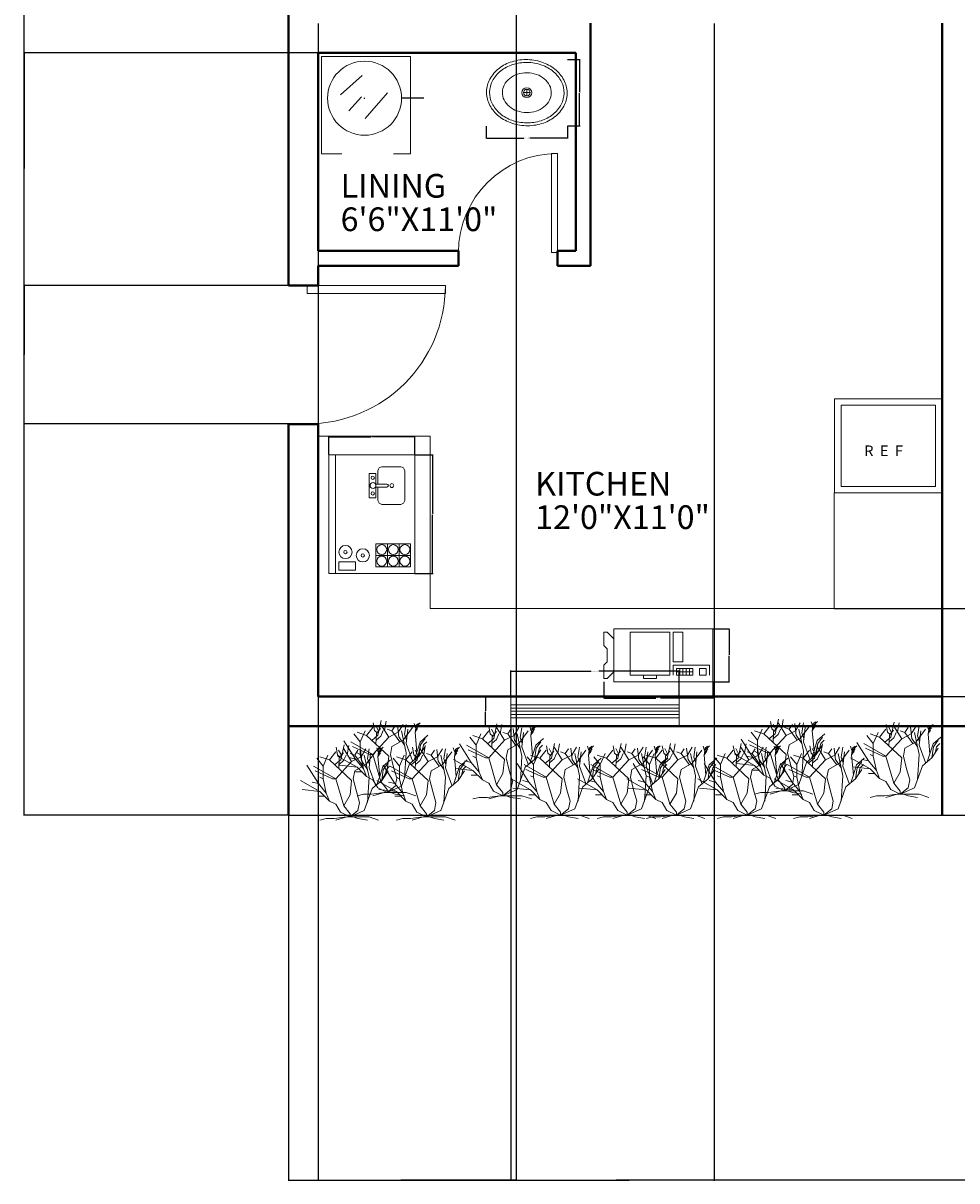
# Model space of a CAD drawing. Units: inches. Extents: x 12978 to 13669, y 46550 to 47327.
# Tile 1 of 5: x 12979 to 13262, y 46550 to 46901. Entities that reach past the tile are written whole.
import ezdxf

# ---------------------------------------------------------------- set-up
doc = ezdxf.new("R2010")
doc.units = ezdxf.units.IN
for name, color, linetype, lineweight in [('A-ANNO-DIMS', 2, 'Continuous', 18), ('A-AREA-IDEN', 1, 'Continuous', 18), ('A-EQPM', 8, 'Continuous', 18), ('A-FLOR-CASE', 8, 'Continuous', 20), ('A-FLOR-FIXT', 9, 'Continuous', 18), ('A-FLOR-OTLN', 7, 'Continuous', 25), ('door', 4, 'Continuous', 20), ('L-PLNT-TREE', 94, 'Continuous', 13), ('text', 1, 'Continuous', 18), ('wall', 7, 'Continuous', 40), ('window', 1, 'Continuous', 18)]:
    doc.layers.add(name, color=color, linetype=linetype, lineweight=lineweight)
doc.styles.get("Standard").update_dxf_attribs({"font": 'arial.ttf'})
doc.dimstyles.get("Standard").update_dxf_attribs({"dimtxt": 0.18, "dimasz": 0.18, "dimexe": 0.18, "dimexo": 0.0625, "dimgap": 0.09, "dimtad": 0, "dimtih": 1, "dimtoh": 1, "dimdec": 4, "dimzin": 0, "dimdsep": 46, "dimtxsty": 'Standard', "dimcen": 0.09, "dimadec": 0, "dimazin": 0, "dimtfac": 1, "dimtdec": 4, "dimtofl": 0, "dimtmove": 0, "dimatfit": 3, "dimfxl": 1, "dimtolj": 1, "dimtzin": 0, "dimarcsym": 0})

# ---------------------------------------------------------------- blocks, each defined once
blk = doc.blocks.new('*U2')
for p, q in [((0, 0), (0, -100)), ((750, 0), (750, -100))]:
    blk.add_line(p, q)
blk.add_lwpolyline([(0, 0), (0, 750), (43.75, 750), (43.75, 0)], close=True)
blk.add_arc((0, 0), 750, 0, 90)
blk = doc.blocks.new('Sink - Oval top')
for p, q in [((-1, 0), (1, 0)), ((0, 1), (0, -1))]:
    blk.add_line(p, q)
for points in [[(-12.23, 0.39, 0.117634), (-11.46, -3.36, 0.104469), (-8.88, -6.8, 0.090016), (-5.08, -9.07, 0.08192), (-0.32, -10.02, 0.08192), (4.49, -9.38, 0.090016), (8.42, -7.36, 0.104469), (11.22, -4.09, 0.117634), (12.23, -0.39, 0.117634), (11.46, 3.36, 0.104469), (8.88, 6.8, 0.090016), (5.08, 9.07, 0.08192), (0.32, 10.02, 0.08192), (-4.49, 9.38, 0.090016), (-8.42, 7.36, 0.104469), (-11.22, 4.09, 0.117634)], [(-11.29, 0.16, 0.118622), (-10.52, -3.25, 0.104678), (-8.07, -6.36, 0.089562), (-4.54, -8.37, 0.081185), (-0.13, -9.15, 0.081185), (4.3, -8.49, 0.089562), (7.89, -6.58, 0.104678), (10.42, -3.55, 0.118622), (11.29, -0.16, 0.118622), (10.52, 3.25, 0.104678), (8.07, 6.36, 0.089562), (4.54, 8.37, 0.081185), (0.13, 9.15, 0.081185), (-4.3, 8.49, 0.089562), (-7.89, 6.58, 0.104678), (-10.42, 3.55, 0.118622)], [(-7.42, 0.08, 0.118283), (-6.91, -2.17, 0.104607), (-5.29, -4.21, 0.089718), (-2.97, -5.53, 0.081436), (-0.07, -6.04, 0.081436), (2.84, -5.59, 0.089718), (5.2, -4.33, 0.104607), (6.86, -2.32, 0.118283), (7.42, -0.08, 0.118283), (6.91, 2.17, 0.104607), (5.29, 4.21, 0.089718), (2.97, 5.53, 0.081436), (0.07, 6.04, 0.081436), (-2.84, 5.59, 0.089718), (-5.2, 4.33, 0.104607), (-6.86, 2.32, 0.118283)]]:
    blk.add_lwpolyline(points, format="xyb", close=True)
for radius in [1.5, 1]:
    blk.add_circle((0, 0), radius)
blk = doc.blocks.new('Wet Bar')
for p, q in [((0, 0), (36, 0)), ((0, -26), (0, 0)), ((36, 0), (36, -26)), ((0, -2), (36, -2)), ((3.5, -3), (1, -3)), ((1, -3), (1, -8)), ((3.5, -8), (3.5, -3)), ((1, -8), (3.5, -8)), ((2, -14.25), (9, -14.25)), ((2, -24.75), (2, -14.25)), ((5.5, -14.25), (5.5, -24.75)), ((9, -14.25), (9, -24.75)), ((26.2, -17.55), (26.2, -14.1284)), ((27.1001, -17.55), (27.1001, -14.1284)), ((2, -17.75), (9, -17.75)), ((9, -21.25), (2, -21.25)), ((36, -26), (0, -26)), ((9, -24.75), (2, -24.75))]:
    blk.add_line(p, q)
for points in [[(26.2, -14.25), (22.95, -14.25), (22.95, -12.2), (26.75, -12.2)], [(26.7487, -12.2), (30.3501, -12.2), (30.3501, -14.25), (27.1001, -14.25)], [(20.95, -21.75), (20.95, -16.05)], [(22.15, -14.85), (26.2, -14.85)], [(27.1001, -14.85), (31.15, -14.85)], [(32.3501, -16.05), (32.3501, -21.75)], [(31.15, -22.95), (22.15, -22.95)]]:
    blk.add_lwpolyline(points)
for centre, radius in [((6.5, -5), 2), ((6.5, -5), 0.5), ((5.5, -10.25), 2), ((5.5, -10.25), 0.5), ((24.25, -13.25), 0.5), ((26.65, -13.35), 0.9), ((29, -13.25), 0.5), ((3.75, -16), 1.5), ((7.25, -16), 1.5), ((3.75, -19.5), 1.5), ((7.25, -19.5), 1.5), ((26.65, -19.05), 0.6), ((3.75, -23), 1.5), ((7.25, -23), 1.5)]:
    blk.add_circle(centre, radius)
for centre, radius, start, end in [((22.2251, -16.125), 1.2772, 93.36646, 176.6335), ((31.075, -16.125), 1.2772, 3.366461, 86.63354), ((26.65, -17.55), 0.45, 180, 0), ((22.2251, -21.675), 1.2772, 183.3665, 266.6335), ((31.075, -21.675), 1.2772, 273.3665, 356.6335)]:
    blk.add_arc(centre, radius, start, end)
blk = doc.blocks.new('Copy Machine')
for p, q in [((0, 0), (0, -16)), ((30, 0), (0, 0)), ((30, -16), (30, 0)), ((-3, -1), (-3, -5)), ((-2, -1), (-3, -1)), ((0, -3), (-2, -1)), ((5, -1), (5, -14)), ((17, -1), (5, -1)), ((17, -14), (17, -1)), ((18, -1), (18, -10)), ((21, -1), (18, -1)), ((21, -10), (21, -1)), ((-3, -5), (-2, -6)), ((-2, -10), (-2, -6)), ((-3, -11), (-2, -10)), ((18, -10), (21, -10)), ((-3, -15), (-3, -11)), ((0, -13), (-2, -15)), ((5, -14), (17, -14)), ((9, -14), (9, -15)), ((13, -15), (13, -14)), ((18, -14), (18, -11)), ((18, -11), (29, -11)), ((24, -12), (19, -12)), ((19, -12), (19, -14)), ((24, -13), (19, -13)), ((19, -14), (24, -14)), ((20, -12), (20, -14)), ((21, -14), (21, -12)), ((22, -12), (22, -14)), ((23, -14), (23, -12)), ((24, -14), (24, -12)), ((28, -12), (26, -12)), ((26, -12), (26, -14)), ((26, -14), (28, -14)), ((28, -14), (28, -12)), ((29, -11), (29, -14)), ((-2, -15), (-3, -15)), ((0, -16), (30, -16)), ((9, -15), (13, -15))]:
    blk.add_line(p, q)
blk = doc.blocks.new('*U13')
for p, q in [((-12.471, 19.775), (-12.898, 22.044)), ((-11.28, 19.619), (-12.104, 21.184)), ((-11.433, 18.289), (-10.457, 22.749)), ((-8.16, 17.76), (-10.56, 21.6)), ((-9.48, 19.775), (-8.992, 22.592)), ((-7.2, 19.68), (-6.24, 21.12)), ((-5.086, 17.741), (-5.513, 21.34)), ((-5.28, 19.2), (-3.84, 21.6)), ((-3.377, 18.602), (-2.888, 21.575)), ((-0.508, 21.888), (-0.081, 20.558)), ((-0.203, 19.149), (0.102, 21.34)), ((-0.02, 20.01), (0.896, 21.105)), ((0.041, 20.714), (1.384, 22.044)), ((0.102, 21.34), (0.835, 21.888)), ((-16.8, 16.32), (-18.72, 18.72)), ((-14.88, 18.24), (-17.76, 19.2)), ((-16.8, 16.32), (-15.36, 19.68)), ((-14.88, 18.24), (-12.96, 20.64)), ((-8.16, 12), (-14.88, 18.24)), ((-13.325, 16.724), (-11.433, 18.289)), ((-12.96, 12.48), (-8.16, 17.76)), ((-11.677, 19.071), (-12.471, 19.775)), ((-12.043, 15.628), (-11.921, 18.836)), ((-11.982, 16.802), (-10.579, 18.054)), ((-11.921, 18.836), (-10.64, 20.401)), ((-10.579, 18.054), (-9.846, 19.697)), ((-7.2, 19.68), (-8.64, 20.16)), ((-8.16, 17.76), (-5.28, 19.2)), ((-4.8, 16.32), (-7.2, 19.68)), ((-3.377, 15.315), (-5.086, 17.819)), ((-2.88, 12.96), (-4.32, 19.68)), ((-3.84, 16.8), (-0.96, 20.64)), ((-2.766, 16.802), (-3.377, 18.602)), ((-2.88, 15.84), (-2.4, 20.16)), ((0.346, 13.203), (-0.203, 19.149)), ((-0.142, 19.384), (0.59, 20.401)), ((1.323, 16.254), (3.642, 18.289)), ((-18.24, 11.04), (-21.755, 16.655)), ((-12.96, 12.48), (-19.68, 16.32)), ((-13.92, 12.48), (-19.2, 14.88)), ((-16.8, 12.48), (-16.8, 16.32)), ((-7.68, 12.48), (-7.2, 14.88)), ((-7.2, 14.88), (-3.84, 16.8)), ((-0.96, 10.56), (-2.88, 15.84)), ((0.346, 13.203), (1.323, 16.254)), ((0.96, 12), (1.44, 15.36)), ((0.96, 12), (2.88, 14.88)), ((1.44, 15.36), (2.88, 17.28)), ((1.92, 13.44), (2.4, 15.36)), ((2.4, 15.36), (3.36, 16.32)), ((-17.76, 8.64), (-23.663, 11.961)), ((-18.24, 11.04), (-20.16, 11.52)), ((-15.84, 8.16), (-18.24, 11.04)), ((-16.8, 12.48), (-17.76, 12.96)), ((-15.84, 8.16), (-16.8, 12.48)), ((-12.96, 12.48), (-13.92, 12.48)), ((-10.56, 4.32), (-12.96, 12.48)), ((-8.64, 7.68), (-8.16, 12)), ((-6.72, 8.64), (-7.68, 12.48)), ((-3.36, 5.28), (-2.88, 12.96)), ((-1.92, 9.6), (0.96, 12)), ((-0.48, 10.8), (0.346, 13.203)), ((-17.76, 8.64), (-23.128, 9.222)), ((-16.32, 7.2), (-18.24, 7.2)), ((-14.88, 5.76), (-17.76, 8.64)), ((-14.88, 5.76), (-15.84, 8.16)), ((-10.56, 4.32), (-8.64, 7.68)), ((-5.76, 5.28), (-6.72, 8.64)), ((-4.32, 2.88), (-1.92, 9.6)), ((-12.96, 4.8), (-14.88, 5.76)), ((-11.52, 2.4), (-12.96, 4.8)), ((-8.64, 1.92), (-10.56, 4.32)), ((-6.24, 2.88), (-5.76, 5.28)), ((-15.84, 0.48), (-17.76, 0)), ((-13.44, 0.48), (-15.84, 0.48)), ((-9.6, 0.96), (-13.44, 0.48)), ((-9.6, 0.96), (-12.96, 0)), ((-8.64, 0.96), (-11.52, 2.4)), ((-9.6, 0.96), (-7.68, 0.96)), ((-8.64, 0.96), (-4.32, 2.88)), ((-8.64, 0.96), (-6.24, 2.88)), ((-8.64, 0.96), (-8.64, 1.92)), ((-8.64, 0.96), (-2.88, 0.96)), ((-7.68, 0.96), (-6.24, 0.48)), ((-6.24, 0.48), (-3.36, 0)), ((-2.88, 0.96), (0, 0))]:
    blk.add_line(p, q)
blk = doc.blocks.new('WINDOW-51')
for p, q in [((0, 0), (0, 9)), ((51.08, 0), (51.08, 9)), ((0, 6.5), (51.08, 6.5)), ((0, 5.5), (51.08, 5.5)), ((0, 4.5), (51.08, 4.5)), ((0, 3.5), (51.08, 3.5)), ((0, 2.5), (51.08, 2.5))]:
    blk.add_line(p, q)
blk = doc.blocks.new('*D43')
at = {"layer": 'A-ANNO-DIMS', "color": 0, "lineweight": -2, "transparency": 16777216}
for p, q in [((13097.3, 46769.89), (13102.82, 46769.89)), ((13102.64, 46769.71), (13102.64, 46752.07)), ((13102.64, 46734.07), (13102.64, 46751.7)), ((13097.3, 46733.89), (13102.82, 46733.89))]:
    blk.add_line(p, q, dxfattribs=at)
at = {"layer": 'A-ANNO-DIMS', "color": 0, "transparency": 16777216}
for points in [[(13102.61, 46769.71), (13102.67, 46769.71), (13102.64, 46769.89)], [(13102.61, 46734.07), (13102.67, 46734.07), (13102.64, 46733.89)]]:
    blk.add_solid(points, dxfattribs=at)
at = {"layer": 'Defpoints', "color": 0, "transparency": 16777216}
for p in [(13097.24, 46769.89), (13102.64, 46769.89), (13097.24, 46733.89)]:
    blk.add_point(p, dxfattribs=at)
at = {"layer": 'A-ANNO-DIMS', "color": 0, "transparency": 16777216, "insert": (13102.64, 46751.89), "char_height": 0.18, "attachment_point": 5}
blk.add_mtext('\\A1;BAR 36', dxfattribs=at)
blk = doc.blocks.new('*D44')
at = {"layer": 'A-ANNO-DIMS', "color": 0, "lineweight": -2, "transparency": 16777216}
for p, q in [((13071.24, 46769.95), (13071.24, 46775.47)), ((13071.42, 46775.29), (13084.01, 46775.29)), ((13097.06, 46775.29), (13084.46, 46775.29)), ((13097.24, 46769.95), (13097.24, 46775.47))]:
    blk.add_line(p, q, dxfattribs=at)
at = {"layer": 'A-ANNO-DIMS', "color": 0, "transparency": 16777216}
for points in [[(13071.42, 46775.32), (13071.42, 46775.26), (13071.24, 46775.29)], [(13097.06, 46775.32), (13097.06, 46775.26), (13097.24, 46775.29)]]:
    blk.add_solid(points, dxfattribs=at)
at = {"layer": 'Defpoints', "color": 0, "transparency": 16777216}
for p in [(13071.24, 46775.29), (13071.24, 46769.89), (13097.24, 46769.89)]:
    blk.add_point(p, dxfattribs=at)
at = {"layer": 'A-ANNO-DIMS', "color": 0, "transparency": 16777216, "insert": (13084.24, 46775.29), "char_height": 0.18, "attachment_point": 5}
blk.add_mtext('\\A1;26', dxfattribs=at)
blk = doc.blocks.new('*D45')
at = {"layer": 'A-ANNO-DIMS', "color": 0, "lineweight": -2, "transparency": 16777216}
for p, q in [((13154.51, 46701.03), (13154.51, 46695.97)), ((13187.51, 46701.03), (13187.51, 46695.97)), ((13154.69, 46696.15), (13170.28, 46696.15)), ((13187.33, 46696.15), (13171.75, 46696.15))]:
    blk.add_line(p, q, dxfattribs=at)
at = {"layer": 'A-ANNO-DIMS', "color": 0, "transparency": 16777216}
for points in [[(13154.69, 46696.18), (13154.69, 46696.12), (13154.51, 46696.15)], [(13187.33, 46696.18), (13187.33, 46696.12), (13187.51, 46696.15)]]:
    blk.add_solid(points, dxfattribs=at)
at = {"layer": 'Defpoints', "color": 0, "transparency": 16777216}
for p in [(13154.51, 46701.1), (13187.51, 46701.1), (13187.51, 46696.15)]:
    blk.add_point(p, dxfattribs=at)
at = {"layer": 'A-ANNO-DIMS', "color": 0, "transparency": 16777216, "insert": (13171.01, 46696.15), "char_height": 0.18, "attachment_point": 5}
blk.add_mtext('\\A1;COPIER 33', dxfattribs=at)
blk = doc.blocks.new('*D46')
at = {"layer": 'A-ANNO-DIMS', "color": 0, "lineweight": -2, "transparency": 16777216}
for p, q in [((13187.57, 46717.1), (13192.64, 46717.1)), ((13192.46, 46716.92), (13192.46, 46709.28)), ((13192.46, 46701.28), (13192.46, 46708.91)), ((13187.57, 46701.1), (13192.64, 46701.1))]:
    blk.add_line(p, q, dxfattribs=at)
at = {"layer": 'A-ANNO-DIMS', "color": 0, "transparency": 16777216}
for points in [[(13192.43, 46716.92), (13192.49, 46716.92), (13192.46, 46717.1)], [(13192.43, 46701.28), (13192.49, 46701.28), (13192.46, 46701.1)]]:
    blk.add_solid(points, dxfattribs=at)
at = {"layer": 'Defpoints', "color": 0, "transparency": 16777216}
for p in [(13187.51, 46717.1), (13192.46, 46717.1), (13187.51, 46701.1)]:
    blk.add_point(p, dxfattribs=at)
at = {"layer": 'A-ANNO-DIMS', "color": 0, "transparency": 16777216, "insert": (13192.46, 46709.1), "char_height": 0.18, "attachment_point": 5}
blk.add_mtext('\\A1;16', dxfattribs=at)
blk = doc.blocks.new('*D47')
at = {"layer": 'A-ANNO-DIMS', "color": 0, "lineweight": -2, "transparency": 16777216}
for p, q in [((13118.92, 46869.44), (13118.92, 46865.64)), ((13143.47, 46869.44), (13143.47, 46865.64)), ((13119.1, 46865.82), (13130.26, 46865.82)), ((13143.29, 46865.82), (13132.13, 46865.82))]:
    blk.add_line(p, q, dxfattribs=at)
at = {"layer": 'A-ANNO-DIMS', "color": 0, "transparency": 16777216}
for points in [[(13119.1, 46865.85), (13119.1, 46865.79), (13118.92, 46865.82)], [(13143.29, 46865.85), (13143.29, 46865.79), (13143.47, 46865.82)]]:
    blk.add_solid(points, dxfattribs=at)
at = {"layer": 'Defpoints', "color": 0, "transparency": 16777216}
for p in [(13118.92, 46869.51), (13143.47, 46869.51), (13143.47, 46865.82)]:
    blk.add_point(p, dxfattribs=at)
at = {"layer": 'A-ANNO-DIMS', "color": 0, "transparency": 16777216, "insert": (13131.19, 46865.82), "char_height": 0.18, "attachment_point": 5}
blk.add_mtext('\\A1;BASIN 25 TYP.', dxfattribs=at)
blk = doc.blocks.new('*D48')
at = {"layer": 'A-ANNO-DIMS', "color": 0, "lineweight": -2, "transparency": 16777216}
for p, q in [((13143.53, 46889.64), (13147.33, 46889.64)), ((13147.15, 46889.46), (13147.15, 46879.76)), ((13147.15, 46869.69), (13147.15, 46879.39)), ((13143.53, 46869.51), (13147.33, 46869.51))]:
    blk.add_line(p, q, dxfattribs=at)
at = {"layer": 'A-ANNO-DIMS', "color": 0, "transparency": 16777216}
for points in [[(13147.12, 46889.46), (13147.18, 46889.46), (13147.15, 46889.64)], [(13147.12, 46869.69), (13147.18, 46869.69), (13147.15, 46869.51)]]:
    blk.add_solid(points, dxfattribs=at)
at = {"layer": 'Defpoints', "color": 0, "transparency": 16777216}
for p in [(13143.47, 46889.64), (13147.15, 46889.64), (13143.47, 46869.51)]:
    blk.add_point(p, dxfattribs=at)
at = {"layer": 'A-ANNO-DIMS', "color": 0, "transparency": 16777216, "insert": (13147.15, 46879.58), "char_height": 0.18, "attachment_point": 5}
blk.add_mtext('\\A1;20 TYP.', dxfattribs=at)
blk = doc.blocks.new('*D49')
at = {"layer": 'A-ANNO-DIMS', "color": 0, "lineweight": -2, "transparency": 16777216}
for p, q in [((13126.32, 46696.7), (13126.32, 46704.48)), ((13126.5, 46704.3), (13150.74, 46704.3)), ((13177.22, 46704.3), (13152.98, 46704.3)), ((13177.4, 46696.7), (13177.4, 46704.48))]:
    blk.add_line(p, q, dxfattribs=at)
at = {"layer": 'A-ANNO-DIMS', "color": 0, "transparency": 16777216}
for points in [[(13126.5, 46704.33), (13126.5, 46704.27), (13126.32, 46704.3)], [(13177.22, 46704.33), (13177.22, 46704.27), (13177.4, 46704.3)]]:
    blk.add_solid(points, dxfattribs=at)
at = {"layer": 'Defpoints', "color": 0, "transparency": 16777216}
for p in [(13177.4, 46704.3), (13126.32, 46696.63), (13177.4, 46696.63)]:
    blk.add_point(p, dxfattribs=at)
at = {"layer": 'A-ANNO-DIMS', "color": 0, "transparency": 16777216, "insert": (13151.86, 46704.3), "char_height": 0.18, "attachment_point": 5}
blk.add_mtext('\\A1;WINDOW 51 TYP.', dxfattribs=at)
blk = doc.blocks.new('*D50')
at = {"layer": 'A-ANNO-DIMS', "color": 0, "lineweight": -2, "transparency": 16777216}
for p, q in [((13126.26, 46696.63), (13118.48, 46696.63)), ((13118.66, 46696.45), (13118.66, 46692.32)), ((13118.66, 46687.81), (13118.66, 46691.95)), ((13126.26, 46687.63), (13118.48, 46687.63))]:
    blk.add_line(p, q, dxfattribs=at)
at = {"layer": 'A-ANNO-DIMS', "color": 0, "transparency": 16777216}
for points in [[(13118.63, 46696.45), (13118.69, 46696.45), (13118.66, 46696.63)], [(13118.63, 46687.81), (13118.69, 46687.81), (13118.66, 46687.63)]]:
    blk.add_solid(points, dxfattribs=at)
at = {"layer": 'Defpoints', "color": 0, "transparency": 16777216}
for p in [(13118.66, 46696.63), (13126.32, 46696.63), (13126.32, 46687.63)]:
    blk.add_point(p, dxfattribs=at)
at = {"layer": 'A-ANNO-DIMS', "color": 0, "transparency": 16777216, "insert": (13118.66, 46692.13), "char_height": 0.18, "attachment_point": 5}
blk.add_mtext('\\A1;9 TYP.', dxfattribs=at)
blk = doc.blocks.new('*D52')
at = {"layer": 'A-ANNO-DIMS', "color": 0, "lineweight": -2, "transparency": 16777216}
for p, q in [((13058.94, 47266.63), (12978.69, 47266.63)), ((12978.87, 47266.45), (12978.87, 46963.82)), ((12978.87, 46660.81), (12978.87, 46963.45)), ((13058.94, 46660.63), (12978.69, 46660.63))]:
    blk.add_line(p, q, dxfattribs=at)
at = {"layer": 'A-ANNO-DIMS', "color": 0, "transparency": 16777216}
for points in [[(12978.84, 47266.45), (12978.9, 47266.45), (12978.87, 47266.63)], [(12978.84, 46660.81), (12978.9, 46660.81), (12978.87, 46660.63)]]:
    blk.add_solid(points, dxfattribs=at)
at = {"layer": 'Defpoints', "color": 0, "transparency": 16777216}
for p in [(12978.87, 47266.63), (13059.01, 47266.63), (13059.01, 46660.63)]:
    blk.add_point(p, dxfattribs=at)
at = {"layer": 'A-ANNO-DIMS', "color": 0, "transparency": 16777216, "insert": (12978.87, 46963.63), "char_height": 0.18, "attachment_point": 5}
blk.add_mtext('\\A1;606', dxfattribs=at)
blk = doc.blocks.new('*D60')
at = {"layer": 'A-ANNO-DIMS', "color": 0, "lineweight": -2, "transparency": 16777216}
for p, q in [((13059.005025, 46660.571951), (13059.005025, 46549.877451)), ((13266.005025, 46660.571951), (13266.005025, 46549.877451)), ((13059.185025, 46550.057451), (13162.214643, 46550.057451)), ((13265.825025, 46550.057451), (13162.795407, 46550.057451))]:
    blk.add_line(p, q, dxfattribs=at)
at = {"layer": 'A-ANNO-DIMS', "color": 0, "transparency": 16777216}
for points in [[(13059.185025, 46550.087451), (13059.185025, 46550.027451), (13059.005025, 46550.057451)], [(13265.825025, 46550.087451), (13265.825025, 46550.027451), (13266.005025, 46550.057451)]]:
    blk.add_solid(points, dxfattribs=at)
at = {"layer": 'Defpoints', "color": 0, "transparency": 16777216}
for p in [(13059.005025, 46660.634451), (13266.005025, 46660.634451), (13266.005025, 46550.057451)]:
    blk.add_point(p, dxfattribs=at)
at = {"layer": 'A-ANNO-DIMS', "color": 0, "transparency": 16777216, "insert": (13162.505025, 46550.057451), "char_height": 0.18, "attachment_point": 5}
blk.add_mtext('\\A1;207', dxfattribs=at)
blk = doc.blocks.new('*D70')
at = {"layer": 'A-ANNO-DIMS', "color": 0, "lineweight": -2, "transparency": 16777216}
for p, q in [((13128.01, 46951.57), (13128.01, 46549.88)), ((13068.01, 46900.57), (13068.01, 46549.88)), ((13068.19, 46550.06), (13097.79, 46550.06)), ((13127.83, 46550.06), (13098.22, 46550.06))]:
    blk.add_line(p, q, dxfattribs=at)
at = {"layer": 'A-ANNO-DIMS', "color": 0, "transparency": 16777216}
for points in [[(13068.19, 46550.09), (13068.19, 46550.03), (13068.01, 46550.06)], [(13127.83, 46550.09), (13127.83, 46550.03), (13128.01, 46550.06)]]:
    blk.add_solid(points, dxfattribs=at)
at = {"layer": 'Defpoints', "color": 0, "transparency": 16777216}
for p in [(13128.01, 46951.63), (13068.01, 46900.63), (13128.01, 46550.06)]:
    blk.add_point(p, dxfattribs=at)
at = {"layer": 'A-ANNO-DIMS', "color": 0, "transparency": 16777216, "insert": (13098.01, 46550.06), "char_height": 0.18, "attachment_point": 5}
blk.add_mtext('\\A1;60', dxfattribs=at)
blk = doc.blocks.new('*D71')
at = {"layer": 'A-ANNO-DIMS', "color": 0, "lineweight": -2, "transparency": 16777216}
for p, q in [((13128.01, 46950.07), (13128.01, 46549.88)), ((13188.01, 46900.57), (13188.01, 46549.88)), ((13128.19, 46550.06), (13157.79, 46550.06)), ((13187.83, 46550.06), (13158.22, 46550.06))]:
    blk.add_line(p, q, dxfattribs=at)
at = {"layer": 'A-ANNO-DIMS', "color": 0, "transparency": 16777216}
for points in [[(13128.19, 46550.09), (13128.19, 46550.03), (13128.01, 46550.06)], [(13187.83, 46550.09), (13187.83, 46550.03), (13188.01, 46550.06)]]:
    blk.add_solid(points, dxfattribs=at)
at = {"layer": 'Defpoints', "color": 0, "transparency": 16777216}
for p in [(13128.01, 46950.13), (13188.01, 46900.63), (13188.01, 46550.06)]:
    blk.add_point(p, dxfattribs=at)
at = {"layer": 'A-ANNO-DIMS', "color": 0, "transparency": 16777216, "insert": (13158.01, 46550.06), "char_height": 0.18, "attachment_point": 5}
blk.add_mtext('\\A1;60', dxfattribs=at)
blk = doc.blocks.new('*D75')
at = {"layer": 'A-ANNO-DIMS', "color": 0, "lineweight": -2, "transparency": 16777216}
for p, q in [((13067.94, 46891.63), (12978.69, 46891.63)), ((12978.87, 46891.45), (12978.87, 46856.57)), ((12978.87, 46821.31), (12978.87, 46856.2)), ((13058.94, 46821.13), (12978.69, 46821.13))]:
    blk.add_line(p, q, dxfattribs=at)
at = {"layer": 'A-ANNO-DIMS', "color": 0, "transparency": 16777216}
for points in [[(12978.84, 46891.45), (12978.9, 46891.45), (12978.87, 46891.63)], [(12978.84, 46821.31), (12978.9, 46821.31), (12978.87, 46821.13)]]:
    blk.add_solid(points, dxfattribs=at)
at = {"layer": 'Defpoints', "color": 0, "transparency": 16777216}
for p in [(13068.01, 46891.63), (12978.87, 46821.13), (13059.01, 46821.13)]:
    blk.add_point(p, dxfattribs=at)
at = {"layer": 'A-ANNO-DIMS', "color": 0, "transparency": 16777216, "insert": (12978.87, 46856.38), "char_height": 0.18, "attachment_point": 5}
blk.add_mtext('\\A1;70.5', dxfattribs=at)
blk = doc.blocks.new('*D76')
at = {"layer": 'A-ANNO-DIMS', "color": 0, "lineweight": -2, "transparency": 16777216}
for p, q in [((13058.94, 46821.13), (12978.69, 46821.13)), ((12978.87, 46820.95), (12978.87, 46800.36)), ((12978.87, 46779.41), (12978.87, 46800)), ((13058.94, 46779.23), (12978.69, 46779.23))]:
    blk.add_line(p, q, dxfattribs=at)
at = {"layer": 'A-ANNO-DIMS', "color": 0, "transparency": 16777216}
for points in [[(12978.84, 46820.95), (12978.9, 46820.95), (12978.87, 46821.13)], [(12978.84, 46779.41), (12978.9, 46779.41), (12978.87, 46779.23)]]:
    blk.add_solid(points, dxfattribs=at)
at = {"layer": 'Defpoints', "color": 0, "transparency": 16777216}
for p in [(12978.87, 46821.13), (13059.01, 46821.13), (13059.01, 46779.23)]:
    blk.add_point(p, dxfattribs=at)
at = {"layer": 'A-ANNO-DIMS', "color": 0, "transparency": 16777216, "insert": (12978.87, 46800.18), "char_height": 0.18, "attachment_point": 5}
blk.add_mtext('\\A1;41.91', dxfattribs=at)
blk = doc.blocks.new('*D77')
at = {"layer": 'A-ANNO-DIMS', "color": 0, "lineweight": -2, "transparency": 16777216}
for p, q in [((13059.01, 46687.57), (13059.01, 46549.88)), ((13126.32, 46687.57), (13126.32, 46549.88)), ((13059.19, 46550.06), (13092.27, 46550.06)), ((13126.14, 46550.06), (13093.06, 46550.06))]:
    blk.add_line(p, q, dxfattribs=at)
at = {"layer": 'A-ANNO-DIMS', "color": 0, "transparency": 16777216}
for points in [[(13059.19, 46550.09), (13059.19, 46550.03), (13059.01, 46550.06)], [(13126.14, 46550.09), (13126.14, 46550.03), (13126.32, 46550.06)]]:
    blk.add_solid(points, dxfattribs=at)
at = {"layer": 'Defpoints', "color": 0, "transparency": 16777216}
for p in [(13059.01, 46687.63), (13126.32, 46687.63), (13126.32, 46550.06)]:
    blk.add_point(p, dxfattribs=at)
at = {"layer": 'A-ANNO-DIMS', "color": 0, "transparency": 16777216, "insert": (13092.66, 46550.06), "char_height": 0.18, "attachment_point": 5}
blk.add_mtext('\\A1;67.32', dxfattribs=at)
blk = doc.blocks.new('*D78')
at = {"layer": 'A-ANNO-DIMS', "color": 0, "lineweight": -2, "transparency": 16777216}
for p, q in [((13224.37, 46723.29), (13669.26, 46723.29)), ((13669.08, 46723.11), (13669.08, 46710.15)), ((13669.08, 46696.81), (13669.08, 46709.78)), ((13257.07, 46696.63), (13669.26, 46696.63))]:
    blk.add_line(p, q, dxfattribs=at)
at = {"layer": 'A-ANNO-DIMS', "color": 0, "transparency": 16777216}
for points in [[(13669.05, 46723.11), (13669.11, 46723.11), (13669.08, 46723.29)], [(13669.05, 46696.81), (13669.11, 46696.81), (13669.08, 46696.63)]]:
    blk.add_solid(points, dxfattribs=at)
at = {"layer": 'Defpoints', "color": 0, "transparency": 16777216}
for p in [(13224.3, 46723.29), (13669.08, 46723.29), (13257.01, 46696.63)]:
    blk.add_point(p, dxfattribs=at)
at = {"layer": 'A-ANNO-DIMS', "color": 0, "transparency": 16777216, "insert": (13669.08, 46709.96), "char_height": 0.18, "attachment_point": 5}
blk.add_mtext('\\A1;26.66', dxfattribs=at)
blk = doc.blocks.new('*D80')
at = {"layer": 'A-ANNO-DIMS', "color": 0, "lineweight": -2, "transparency": 16777216}
for p, q in [((13081.93, 46877.9), (13082.11, 46877.9)), ((13082.02, 46877.81), (13082.02, 46877.99)), ((13099.96, 46877.9), (13093.41, 46877.9))]:
    blk.add_line(p, q, dxfattribs=at)
at = {"layer": 'A-ANNO-DIMS', "color": 0, "transparency": 16777216}
blk.add_solid([(13093.41, 46877.93), (13093.41, 46877.87), (13093.23, 46877.9)], dxfattribs=at)
at = {"layer": 'Defpoints', "color": 0, "transparency": 16777216}
for p in [(13070.8, 46877.9), (13093.23, 46877.9)]:
    blk.add_point(p, dxfattribs=at)
at = {"layer": 'A-ANNO-DIMS', "color": 0, "transparency": 16777216, "insert": (13100.46, 46877.9), "char_height": 0.18, "attachment_point": 5}
blk.add_mtext('\\A1;∅22.43', dxfattribs=at)

msp = doc.modelspace()

# ---------------------------------------------------------------- linework, layer by layer
at = {"layer": 'A-EQPM'}
for p, q in [((13068.9629, 46890.5263), (13095.9528, 46890.5263)), ((13068.9629, 46861.0846), (13068.9629, 46890.5263)), ((13095.9528, 46890.5263), (13095.9528, 46861.0846)), ((13074.6847, 46878.9294), (13081.2861, 46884.7902)), ((13082.1657, 46871.7177), (13089.0061, 46879.5343)), ((13077.2961, 46874.0393), (13081.0642, 46878.2661)), ((13075.177, 46861.0846), (13068.9629, 46861.0846)), ((13095.9528, 46861.0846), (13090.8372, 46861.0846))]:
    msp.add_line(p, q, dxfattribs=at)
for points in [[(13257.005, 46758.2817), (13224.441, 46758.2817), (13224.441, 46786.8478), (13257.005, 46786.8478)], [(13255.005, 46760.2817), (13226.441, 46760.2817), (13226.441, 46784.8478), (13255.005, 46784.8478)]]:
    msp.add_lwpolyline(points, close=True, dxfattribs=at)
msp.add_circle((13082.0195, 46877.9038), 11.2155, dxfattribs=at)
at = {"layer": 'A-FLOR-CASE'}
for p, q in [((13068.005, 46775.4644), (13101.8868, 46775.4644)), ((13101.8868, 46775.4644), (13101.8868, 46723.2923)), ((13224.303, 46723.2923), (13224.303, 46758.2817)), ((13224.303, 46758.2817), (13257.005, 46758.2817)), ((13101.8868, 46723.2923), (13224.303, 46723.2923))]:
    msp.add_line(p, q, dxfattribs=at)
at = {"layer": 'A-FLOR-OTLN'}
msp.add_line((13059.005, 46660.6345), (13431.005, 46660.6345), dxfattribs=at)
at = {"layer": 'wall'}
for p, q in [((13059.005, 47266.6345), (13059.005, 46821.1345)), ((13150.505, 46900.6345), (13150.505, 46827.1345)), ((13257.005, 46900.6345), (13257.005, 46660.6345)), ((13068.005, 46891.6345), (13146.005, 46891.6345)), ((13068.005, 46891.6345), (13068.005, 46831.6345)), ((13146.005, 46891.6345), (13146.005, 46831.6345)), ((13068.005, 46831.6345), (13110.4591, 46831.6345)), ((13110.4591, 46831.6345), (13110.4591, 46827.1345)), ((13140.4591, 46831.6345), (13140.4591, 46827.1345)), ((13140.4591, 46831.6345), (13146.005, 46831.6345)), ((13068.005, 46827.1345), (13110.4591, 46827.1345)), ((13068.005, 46827.1345), (13068.005, 46821.1345)), ((13140.4591, 46827.1345), (13150.505, 46827.1345)), ((13068.005, 46821.1345), (13059.005, 46821.1345)), ((13068.005, 46779.1345), (13059.005, 46779.1345)), ((13059.005, 46779.1345), (13059.005, 46660.6345)), ((13068.005, 46779.1345), (13068.005, 46696.6345)), ((13068.005, 46696.6345), (13257.005, 46696.6345)), ((13059.005, 46687.6345), (13266.005, 46687.6345))]:
    msp.add_line(p, q, dxfattribs=at)

# ---------------------------------------------------------------- block references
at = {"layer": 'A-EQPM'}
msp.add_blockref('Copy Machine', (13157.5124, 46717.0965), dxfattribs=at)
at = {"layer": 'A-FLOR-FIXT'}
msp.add_blockref('Sink - Oval top', (13131.1943, 46879.5756), dxfattribs=at)
at = {"layer": 'A-FLOR-FIXT', "rotation": 90}
msp.add_blockref('Wet Bar', (13071.2351, 46733.8856), dxfattribs=at)
at = {"layer": 'door', "xscale": -0.0400000000000011, "yscale": 0.0400000000000011, "zscale": 0.0400000000000011}
msp.add_blockref('*U2', (13140.4591, 46831.1345), dxfattribs=at)
at = {"layer": 'door', "xscale": 0.0558759688399716, "yscale": 0.0558759688399716, "zscale": 0.0558759688399716, "rotation": 270}
msp.add_blockref('*U2', (13064.5926, 46821.1345), dxfattribs=at)
at = {"layer": 'L-PLNT-TREE'}
for p in [(13097.5171, 46666.5758), (13217.8995, 46667.0558), (13132.5938, 46665.5843), (13252.9762, 46666.0643), (13150.0626, 46659.6745), (13170.2482, 46659.6745), (13185.1393, 46659.6745), (13206.6486, 46659.6745), (13229.8124, 46659.6745), (13086.2662, 46659.1945), (13109.43, 46659.1945)]:
    msp.add_blockref('*U13', p, dxfattribs=at)
at = {"layer": 'window'}
msp.add_blockref('WINDOW-51', (13126.3221, 46687.6345), dxfattribs=at)

# ---------------------------------------------------------------- texts
at = {"layer": 'A-AREA-IDEN'}
for s, height, p in [('LINING', 7.17855, (13074.7579, 46847.7632)), ('6\'6"X11\'0"', 7.17855, (13074.7579, 46837.6247)), ('KITCHEN', 7.17855, (13133.7107, 46757.5045)), ('12\'0"X11\'0"', 7.178549, (13133.7107, 46747.366))]:
    msp.add_text(s, height=height, dxfattribs=at).set_placement(p)
at = {"layer": 'text'}
msp.add_text('R  E  F', height=3.21694, dxfattribs=at).set_placement((13233.4679, 46769.4658))

# ---------------------------------------------------------------- dimensions: what is measured, and where the dimension line sits
at = {"layer": 'A-ANNO-DIMS'}
for base, p1, p2, angle, override, picture, middle in [((12978.8702, 47266.6345), (13059.005, 46660.6345), (13059.005, 47266.6345), 90, {"dimdec": 0, "dimlfac": 1, "dimrnd": 0, "dimzin": 0, "dimdsep": 46, "dimlunit": 2}, '*D52', (12978.8702, 46963.6345)), ((12978.8702, 46821.1345), (13068.005, 46891.6345), (13059.005, 46821.1345), 90, {"dimdec": 1, "dimlfac": 1, "dimrnd": 0, "dimzin": 0, "dimdsep": 46, "dimlunit": 2}, '*D75', (12978.8702, 46856.3845)), ((12978.8702, 46821.1345), (13059.005, 46779.2275), (13059.005, 46821.1345), 90, {"dimdec": 2, "dimlfac": 1, "dimrnd": 0, "dimzin": 0, "dimdsep": 46, "dimlunit": 2}, '*D76', (12978.8702, 46800.181)), ((13071.2351, 46775.2856), (13097.2351, 46769.8856), (13071.2351, 46769.8856), 180, {"dimdec": 0, "dimlfac": 1, "dimrnd": 0, "dimzin": 0, "dimdsep": 46, "dimlunit": 2}, '*D44', (13084.2351, 46775.2856)), ((13669.0793, 46723.2923), (13257.005, 46696.6345), (13224.303, 46723.2923), 90, {"dimdec": 2, "dimlfac": 1, "dimrnd": 0, "dimzin": 0, "dimdsep": 46, "dimlunit": 2}, '*D78', (13669.0793, 46709.9634)), ((13192.4624, 46717.0965), (13187.5124, 46701.0965), (13187.5124, 46717.0965), 90, {"dimdec": 0, "dimlfac": 1, "dimrnd": 0, "dimzin": 0, "dimdsep": 46, "dimlunit": 2}, '*D46', (13192.4624, 46709.0965))]:
    dim = msp.add_linear_dim(base=base, p1=p1, p2=p2, angle=angle, dimstyle='Standard', override=override, dxfattribs=at)
    dim.commit()
    dim.dimension.update_dxf_attribs({"geometry": picture, "text_midpoint": middle})
for base, p1, p2, override, picture, middle in [((13128.005, 46550.0575), (13068.005, 46900.6345), (13128.005, 46951.6345), {"dimdec": 0, "dimlfac": 1, "dimrnd": 0, "dimzin": 0, "dimdsep": 46, "dimlunit": 2}, '*D70', (13098.005, 46550.0575)), ((13188.005, 46550.0575), (13128.005, 46950.1345), (13188.005, 46900.6345), {"dimdec": 0, "dimlfac": 1, "dimrnd": 0, "dimzin": 0, "dimdsep": 46, "dimlunit": 2}, '*D71', (13158.005, 46550.0575)), ((13126.3221, 46550.0575), (13059.005, 46687.6345), (13126.3221, 46687.6345), {"dimdec": 2, "dimlfac": 1, "dimrnd": 0, "dimzin": 0, "dimdsep": 46, "dimlunit": 2}, '*D77', (13092.6636, 46550.0575)), ((13266.005, 46550.0575), (13059.005, 46660.6345), (13266.005, 46660.6345), {"dimdec": 0, "dimlfac": 1, "dimrnd": 0, "dimzin": 0, "dimdsep": 46, "dimlunit": 2}, '*D60', (13162.505, 46550.0575))]:
    dim = msp.add_linear_dim(base=base, p1=p1, p2=p2, dimstyle='Standard', override=override, dxfattribs=at)
    dim.commit()
    dim.dimension.update_dxf_attribs({"geometry": picture, "text_midpoint": middle})
for base, p1, p2, text, picture, middle in [((13147.1523, 46889.6439), (13143.4697, 46869.5073), (13143.4697, 46889.6439), '<> TYP.', '*D48', (13147.1523, 46879.5756)), ((13102.6351, 46769.8856), (13097.2351, 46733.8856), (13097.2351, 46769.8856), 'BAR <>', '*D43', (13102.6351, 46751.8856)), ((13118.6608, 46696.6345), (13126.3221, 46687.6345), (13126.3221, 46696.6345), '<> TYP.', '*D50', (13118.6608, 46692.1345))]:
    dim = msp.add_linear_dim(base=base, p1=p1, p2=p2, angle=90, text=text, dimstyle='Standard', override={"dimdec": 0, "dimlfac": 1, "dimrnd": 0, "dimzin": 0, "dimdsep": 46, "dimlunit": 2}, dxfattribs=at)
    dim.commit()
    dim.dimension.update_dxf_attribs({"geometry": picture, "text_midpoint": middle})
dim = msp.add_diameter_dim_2p(p1=(13070.804, 46877.9036), p2=(13093.2349, 46877.904), dimstyle='Standard', override={"dimdec": 2, "dimlfac": 1, "dimrnd": 0, "dimzin": 0, "dimdsep": 46, "dimlunit": 2}, dxfattribs=at)
dim.commit()
dim.dimension.update_dxf_attribs({"geometry": '*D80', "text_midpoint": (13099.9642, 46877.9041), "dimtype": 163})
for base, p1, p2, text, picture, middle in [((13143.4697, 46865.8247), (13118.9188, 46869.5073), (13143.4697, 46869.5073), 'BASIN <> TYP.', '*D47', (13131.1943, 46865.8247)), ((13177.3974, 46704.2957), (13126.3221, 46696.6345), (13177.3974, 46696.6345), 'WINDOW <> TYP.', '*D49', (13151.8597, 46704.2957)), ((13187.5124, 46696.1465), (13154.5124, 46701.0965), (13187.5124, 46701.0965), 'COPIER <>', '*D45', (13171.0124, 46696.1465))]:
    dim = msp.add_linear_dim(base=base, p1=p1, p2=p2, text=text, dimstyle='Standard', override={"dimdec": 0, "dimlfac": 1, "dimrnd": 0, "dimzin": 0, "dimdsep": 46, "dimlunit": 2}, dxfattribs=at)
    dim.commit()
    dim.dimension.update_dxf_attribs({"geometry": picture, "text_midpoint": middle})

doc.saveas('drawing.dxf')
